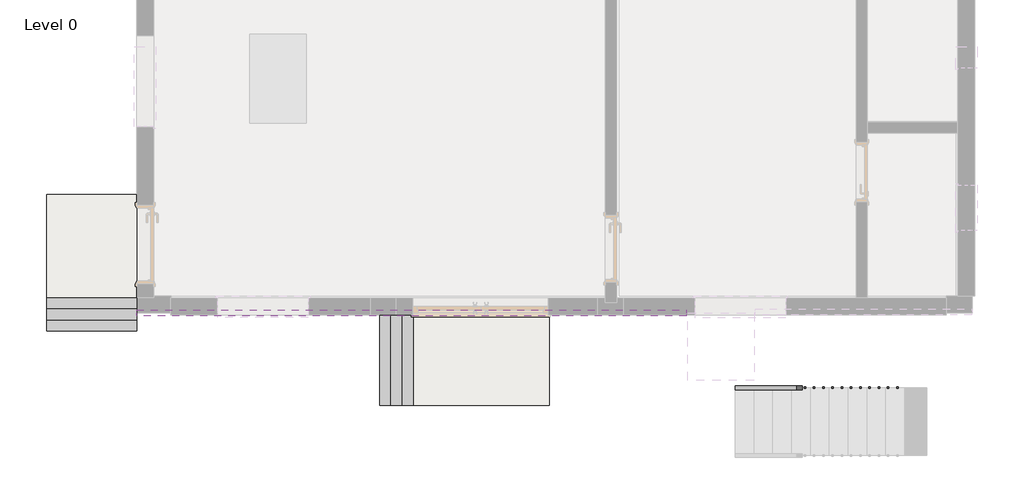
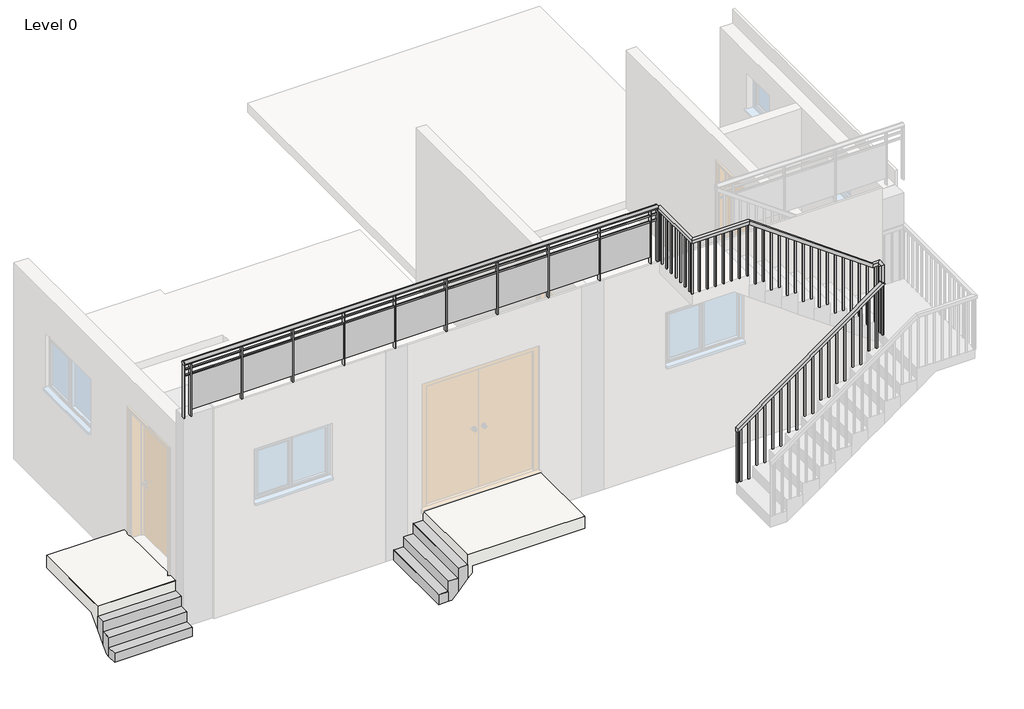
# One storey, part 2 of 3: 2 railings, 2 slabs, 2 stair flights.
"""IFC4 building model written with IfcOpenShell, lengths in millimetres."""

from ifc_helpers import new_model, si_unit, point, frame, origin, place, context, project, spatial, polyline, ellipse_curve, trimmed, outline, extrude, faceted_brep, element, save
from ifc_brep_helpers import plane_surface, extruded_surface, advanced_brep

model = new_model("IFC4")

# Units and contexts
model_context = context("Model", 3, world=origin())
ifc_project = project(units=[si_unit("LENGTHUNIT", "METRE", prefix="MILLI")], contexts=[model_context])

# Site, building, storey
site = spatial("IfcSite", under=ifc_project)
building = spatial("IfcBuilding", under=site)
storey = spatial("IfcBuildingStorey", under=building, Name="Level 0", Elevation=0.0)

# Railings
placement = place(None, origin())
element("IfcRailing", 1, ObjectType="900mm", at=placement, inside=storey, context=model_context, shape_type="SolidModel", body=[
    faceted_brep([(-2174.6019478, -2489.8095641, 610.0312421), (-2174.6019478, -2489.8095641, 548.4309995), (-2174.6019478, -2539.8095641, 548.4309995), (-2174.6019478, -2539.8095641, 610.0312421), (86.3425269, -2489.8095641, 2237.0254162), (86.3425269, -2539.8095641, 2237.0254162), (136.3425269, -2539.8095641, 2211.4055833), (136.3425269, -2489.8095641, 2211.4055833)], [[[0, 1, 2, 3]], [[4, 5, 6, 7]], [[1, 0, 4, 7]], [[2, 1, 7, 6]], [[3, 2, 6, 5]], [[0, 3, 5, 4]]]),
    faceted_brep([(86.3425269, -2513.6043721, 2237.0254162), (86.3425269, -2463.6043721, 2237.0254162), (136.3425269, -2463.6043721, 2211.4055833), (136.3425269, -2513.6043721, 2211.4055833), (86.3425269, -2513.6043721, 2509.7527012), (86.3425269, -2463.6043721, 2459.7527012), (136.3425269, -2463.6043721, 2459.7527012), (136.3425269, -2513.6043721, 2509.7527012), (86.3425269, -2438.6043721, 2509.7527012), (86.3425269, -2438.6043721, 2459.7527012), (136.3425269, -2388.6043721, 2459.7527012), (136.3425269, -2388.6043721, 2509.7527012), (11.3425269, -2438.6043721, 2509.7527012), (-4.7777331, -2438.6043721, 2459.7527012), (-4.7777331, -2388.6043721, 2459.7527012), (11.3425269, -2388.6043721, 2509.7527012), (-1920.6019478, -2438.6043721, 3900.0), (-1936.7222077, -2438.6043721, 3850.0), (-1936.7222077, -2388.6043721, 3850.0), (-1920.6019478, -2388.6043721, 3900.0), (-2838.6867445, -2438.6043721, 3900.0), (-2838.6867445, -2438.6043721, 3850.0), (-2788.6867445, -2388.6043721, 3850.0), (-2788.6867445, -2388.6043721, 3900.0), (-2838.6867445, -1501.447153, 3900.0), (-2788.6867445, -1501.447153, 3900.0), (-2788.6867445, -1501.447153, 3850.0), (-2838.6867445, -1501.447153, 3850.0)], [[[0, 1, 2, 3]], [[1, 0, 4, 5]], [[2, 1, 5, 6]], [[3, 2, 6, 7]], [[0, 3, 7, 4]], [[5, 4, 8, 9]], [[6, 5, 9, 10]], [[7, 6, 10, 11]], [[4, 7, 11, 8]], [[9, 8, 12, 13]], [[10, 9, 13, 14]], [[11, 10, 14, 15]], [[8, 11, 15, 12]], [[13, 12, 16, 17]], [[14, 13, 17, 18]], [[15, 14, 18, 19]], [[12, 15, 19, 16]], [[17, 16, 20, 21]], [[18, 17, 21, 22]], [[19, 18, 22, 23]], [[16, 19, 23, 20]], [[24, 25, 26, 27]], [[21, 20, 24, 27]], [[22, 21, 27, 26]], [[23, 22, 26, 25]], [[20, 23, 25, 24]]]),
    extrude(outline(polyline([(-2803.6867445, -1611.1043721), (-2823.6867445, -1611.1043721), (-2823.6867445, -1591.1043721), (-2803.6867445, -1591.1043721), (-2803.6867445, -1611.1043721)])), frame((0.0, 0.0, 3000.0), z_axis=(0.0, 0.0, 1.0), x_axis=(1.0, 0.0, 0.0)), (0.0, 0.0, 1.0), 850.0),
    extrude(outline(polyline([(-2803.6867445, -1736.1043721), (-2823.6867445, -1736.1043721), (-2823.6867445, -1716.1043721), (-2803.6867445, -1716.1043721), (-2803.6867445, -1736.1043721)])), frame((0.0, 0.0, 3000.0), z_axis=(0.0, 0.0, 1.0), x_axis=(1.0, 0.0, 0.0)), (0.0, 0.0, 1.0), 850.0),
    extrude(outline(polyline([(-2803.6867445, -1861.1043721), (-2823.6867445, -1861.1043721), (-2823.6867445, -1841.1043721), (-2803.6867445, -1841.1043721), (-2803.6867445, -1861.1043721)])), frame((0.0, 0.0, 3000.0), z_axis=(0.0, 0.0, 1.0), x_axis=(1.0, 0.0, 0.0)), (0.0, 0.0, 1.0), 850.0),
    extrude(outline(polyline([(-2803.6867445, -1986.1043721), (-2823.6867445, -1986.1043721), (-2823.6867445, -1966.1043721), (-2803.6867445, -1966.1043721), (-2803.6867445, -1986.1043721)])), frame((0.0, 0.0, 3000.0), z_axis=(0.0, 0.0, 1.0), x_axis=(1.0, 0.0, 0.0)), (0.0, 0.0, 1.0), 850.0),
    extrude(outline(polyline([(-2803.6867445, -2111.1043721), (-2823.6867445, -2111.1043721), (-2823.6867445, -2091.1043721), (-2803.6867445, -2091.1043721), (-2803.6867445, -2111.1043721)])), frame((0.0, 0.0, 3000.0), z_axis=(0.0, 0.0, 1.0), x_axis=(1.0, 0.0, 0.0)), (0.0, 0.0, 1.0), 850.0),
    extrude(outline(polyline([(-2803.6867445, -2236.1043721), (-2823.6867445, -2236.1043721), (-2823.6867445, -2216.1043721), (-2803.6867445, -2216.1043721), (-2803.6867445, -2236.1043721)])), frame((0.0, 0.0, 3000.0), z_axis=(0.0, 0.0, 1.0), x_axis=(1.0, 0.0, 0.0)), (0.0, 0.0, 1.0), 850.0),
    extrude(outline(polyline([(-2803.6867445, -2361.1043721), (-2823.6867445, -2361.1043721), (-2823.6867445, -2341.1043721), (-2803.6867445, -2341.1043721), (-2803.6867445, -2361.1043721)])), frame((0.0, 0.0, 3000.0), z_axis=(0.0, 0.0, 1.0), x_axis=(1.0, 0.0, 0.0)), (0.0, 0.0, 1.0), 850.0),
    extrude(outline(polyline([(-2691.1574731, -2403.6043721), (-2691.1574731, -2423.6043721), (-2711.1574731, -2423.6043721), (-2711.1574731, -2403.6043721), (-2691.1574731, -2403.6043721)])), frame((0.0, 0.0, 3000.0), z_axis=(0.0, 0.0, 1.0), x_axis=(1.0, 0.0, 0.0)), (0.0, 0.0, 1.0), 850.0),
    extrude(outline(polyline([(-2566.1574731, -2403.6043721), (-2566.1574731, -2423.6043721), (-2586.1574731, -2423.6043721), (-2586.1574731, -2403.6043721), (-2566.1574731, -2403.6043721)])), frame((0.0, 0.0, 3000.0), z_axis=(0.0, 0.0, 1.0), x_axis=(1.0, 0.0, 0.0)), (0.0, 0.0, 1.0), 850.0),
    extrude(outline(polyline([(-2441.1574731, -2403.6043721), (-2441.1574731, -2423.6043721), (-2461.1574731, -2423.6043721), (-2461.1574731, -2403.6043721), (-2441.1574731, -2403.6043721)])), frame((0.0, 0.0, 3000.0), z_axis=(0.0, 0.0, 1.0), x_axis=(1.0, 0.0, 0.0)), (0.0, 0.0, 1.0), 850.0),
    extrude(outline(polyline([(-2316.1574731, -2403.6043721), (-2316.1574731, -2423.6043721), (-2336.1574731, -2423.6043721), (-2336.1574731, -2403.6043721), (-2316.1574731, -2403.6043721)])), frame((0.0, 0.0, 3000.0), z_axis=(0.0, 0.0, 1.0), x_axis=(1.0, 0.0, 0.0)), (0.0, 0.0, 1.0), 850.0),
    extrude(outline(polyline([(-2191.1574731, -2403.6043721), (-2191.1574731, -2423.6043721), (-2211.1574731, -2423.6043721), (-2211.1574731, -2403.6043721), (-2191.1574731, -2403.6043721)])), frame((0.0, 0.0, 3000.0), z_axis=(0.0, 0.0, 1.0), x_axis=(1.0, 0.0, 0.0)), (0.0, 0.0, 1.0), 850.0),
    extrude(outline(polyline([(-2066.1574731, -2403.6043721), (-2066.1574731, -2423.6043721), (-2086.1574731, -2423.6043721), (-2086.1574731, -2403.6043721), (-2066.1574731, -2403.6043721)])), frame((0.0, 0.0, 3000.0), z_axis=(0.0, 0.0, 1.0), x_axis=(1.0, 0.0, 0.0)), (0.0, 0.0, 1.0), 850.0),
    extrude(outline(polyline([(-1941.1574731, -2403.6043721), (-1941.1574731, -2423.6043721), (-1961.1574731, -2423.6043721), (-1961.1574731, -2403.6043721), (-1941.1574731, -2403.6043721)])), frame((0.0, 0.0, 3000.0), z_axis=(0.0, 0.0, 1.0), x_axis=(1.0, 0.0, 0.0)), (0.0, 0.0, 1.0), 850.0),
    extrude(outline(polyline([(2817.2239579, -1816.1574731), (3763.2362178, -1816.1574731), (3777.6283817, -1836.1574731), (2817.2239579, -1836.1574731), (2817.2239579, -1816.1574731)])), frame((0.0, -2423.6043721, 0.0), z_axis=(0.0, 1.0, 0.0), x_axis=(0.0, 0.0, 1.0)), (0.0, 0.0, 1.0), 20.0),
    extrude(outline(polyline([(2817.2239579, -1691.1574731), (3673.2851934, -1691.1574731), (3687.6773573, -1711.1574731), (2817.2239579, -1711.1574731), (2817.2239579, -1691.1574731)])), frame((0.0, -2423.6043721, 0.0), z_axis=(0.0, 1.0, 0.0), x_axis=(0.0, 0.0, 1.0)), (0.0, 0.0, 1.0), 20.0),
    extrude(outline(polyline([(2634.4479158, -1566.1574731), (3583.3341689, -1566.1574731), (3597.7263328, -1586.1574731), (2634.4479158, -1586.1574731), (2634.4479158, -1566.1574731)])), frame((0.0, -2423.6043721, 0.0), z_axis=(0.0, 1.0, 0.0), x_axis=(0.0, 0.0, 1.0)), (0.0, 0.0, 1.0), 20.0),
    extrude(outline(polyline([(2634.4479158, -1441.1574731), (3493.3831444, -1441.1574731), (3507.7753083, -1461.1574731), (2634.4479158, -1461.1574731), (2634.4479158, -1441.1574731)])), frame((0.0, -2423.6043721, 0.0), z_axis=(0.0, 1.0, 0.0), x_axis=(0.0, 0.0, 1.0)), (0.0, 0.0, 1.0), 20.0),
    extrude(outline(polyline([(2451.6718737, -1316.1574731), (3403.43212, -1316.1574731), (3417.8242839, -1336.1574731), (2451.6718737, -1336.1574731), (2451.6718737, -1316.1574731)])), frame((0.0, -2423.6043721, 0.0), z_axis=(0.0, 1.0, 0.0), x_axis=(0.0, 0.0, 1.0)), (0.0, 0.0, 1.0), 20.0),
    extrude(outline(polyline([(2451.6718737, -1191.1574731), (3313.4810955, -1191.1574731), (3327.8732594, -1211.1574731), (2451.6718737, -1211.1574731), (2451.6718737, -1191.1574731)])), frame((0.0, -2423.6043721, 0.0), z_axis=(0.0, 1.0, 0.0), x_axis=(0.0, 0.0, 1.0)), (0.0, 0.0, 1.0), 20.0),
    extrude(outline(polyline([(2268.8958316, -1066.1574731), (3223.530071, -1066.1574731), (3237.9222349, -1086.1574731), (2268.8958316, -1086.1574731), (2268.8958316, -1066.1574731)])), frame((0.0, -2423.6043721, 0.0), z_axis=(0.0, 1.0, 0.0), x_axis=(0.0, 0.0, 1.0)), (0.0, 0.0, 1.0), 20.0),
    extrude(outline(polyline([(2268.8958316, -941.1574731), (3133.5790466, -941.1574731), (3147.9712105, -961.1574731), (2268.8958316, -961.1574731), (2268.8958316, -941.1574731)])), frame((0.0, -2423.6043721, 0.0), z_axis=(0.0, 1.0, 0.0), x_axis=(0.0, 0.0, 1.0)), (0.0, 0.0, 1.0), 20.0),
    extrude(outline(polyline([(2086.1197895, -816.1574731), (3043.6280221, -816.1574731), (3058.020186, -836.1574731), (2086.1197895, -836.1574731), (2086.1197895, -816.1574731)])), frame((0.0, -2423.6043721, 0.0), z_axis=(0.0, 1.0, 0.0), x_axis=(0.0, 0.0, 1.0)), (0.0, 0.0, 1.0), 20.0),
    extrude(outline(polyline([(2086.1197895, -691.1574731), (2953.6769976, -691.1574731), (2968.0691615, -711.1574731), (2086.1197895, -711.1574731), (2086.1197895, -691.1574731)])), frame((0.0, -2423.6043721, 0.0), z_axis=(0.0, 1.0, 0.0), x_axis=(0.0, 0.0, 1.0)), (0.0, 0.0, 1.0), 20.0),
    extrude(outline(polyline([(1903.3437474, -566.1574731), (2863.7259732, -566.1574731), (2878.1181371, -586.1574731), (1903.3437474, -586.1574731), (1903.3437474, -566.1574731)])), frame((0.0, -2423.6043721, 0.0), z_axis=(0.0, 1.0, 0.0), x_axis=(0.0, 0.0, 1.0)), (0.0, 0.0, 1.0), 20.0),
    extrude(outline(polyline([(1903.3437474, -441.1574731), (2773.7749487, -441.1574731), (2788.1671126, -461.1574731), (1903.3437474, -461.1574731), (1903.3437474, -441.1574731)])), frame((0.0, -2423.6043721, 0.0), z_axis=(0.0, 1.0, 0.0), x_axis=(0.0, 0.0, 1.0)), (0.0, 0.0, 1.0), 20.0),
    extrude(outline(polyline([(1720.5677053, -316.1574731), (2683.8239242, -316.1574731), (2698.2160881, -336.1574731), (1720.5677053, -336.1574731), (1720.5677053, -316.1574731)])), frame((0.0, -2423.6043721, 0.0), z_axis=(0.0, 1.0, 0.0), x_axis=(0.0, 0.0, 1.0)), (0.0, 0.0, 1.0), 20.0),
    extrude(outline(polyline([(1720.5677053, -191.1574731), (2593.8728998, -191.1574731), (2608.2650637, -211.1574731), (1720.5677053, -211.1574731), (1720.5677053, -191.1574731)])), frame((0.0, -2423.6043721, 0.0), z_axis=(0.0, 1.0, 0.0), x_axis=(0.0, 0.0, 1.0)), (0.0, 0.0, 1.0), 20.0),
    extrude(outline(polyline([(1537.7916632, -66.1574731), (2503.9218753, -66.1574731), (2518.3140392, -86.1574731), (1537.7916632, -86.1574731), (1537.7916632, -66.1574731)])), frame((0.0, -2423.6043721, 0.0), z_axis=(0.0, 1.0, 0.0), x_axis=(0.0, 0.0, 1.0)), (0.0, 0.0, 1.0), 20.0),
    extrude(outline(polyline([(58.8425269, -2403.6043721), (58.8425269, -2423.6043721), (38.8425269, -2423.6043721), (38.8425269, -2403.6043721), (58.8425269, -2403.6043721)])), frame((0.0, 0.0, 1537.7916632), z_axis=(0.0, 0.0, 1.0), x_axis=(1.0, 0.0, 0.0)), (0.0, 0.0, 1.0), 921.9610381),
    extrude(outline(polyline([(121.3425269, -2462.3095641), (101.3425269, -2462.3095641), (101.3425269, -2442.3095641), (121.3425269, -2442.3095641), (121.3425269, -2462.3095641)])), frame((0.0, 0.0, 1355.0156211), z_axis=(0.0, 0.0, 1.0), x_axis=(1.0, 0.0, 0.0)), (0.0, 0.0, 1.0), 1104.7370802),
    extrude(outline(polyline([(2115.3778457, 2.8980522), (1172.2395789, 2.8980522), (1172.2395789, 22.8980522), (2129.7700096, 22.8980522), (2115.3778457, 2.8980522)])), frame((0.0, -2524.8095641, 0.0), z_axis=(0.0, 1.0, 0.0), x_axis=(0.0, 0.0, 1.0)), (0.0, 0.0, 1.0), 20.0),
    extrude(outline(polyline([(2025.4268212, -122.1019478), (1172.2395789, -122.1019478), (1172.2395789, -102.1019478), (2039.8189852, -102.1019478), (2025.4268212, -122.1019478)])), frame((0.0, -2524.8095641, 0.0), z_axis=(0.0, 1.0, 0.0), x_axis=(0.0, 0.0, 1.0)), (0.0, 0.0, 1.0), 20.0),
    extrude(outline(polyline([(1935.4757968, -247.1019478), (989.4635368, -247.1019478), (989.4635368, -227.1019478), (1949.8679607, -227.1019478), (1935.4757968, -247.1019478)])), frame((0.0, -2524.8095641, 0.0), z_axis=(0.0, 1.0, 0.0), x_axis=(0.0, 0.0, 1.0)), (0.0, 0.0, 1.0), 20.0),
    extrude(outline(polyline([(1845.5247723, -372.1019478), (989.4635368, -372.1019478), (989.4635368, -352.1019478), (1859.9169362, -352.1019478), (1845.5247723, -372.1019478)])), frame((0.0, -2524.8095641, 0.0), z_axis=(0.0, 1.0, 0.0), x_axis=(0.0, 0.0, 1.0)), (0.0, 0.0, 1.0), 20.0),
    extrude(outline(polyline([(1755.5737478, -497.1019478), (806.6874947, -497.1019478), (806.6874947, -477.1019478), (1769.9659118, -477.1019478), (1755.5737478, -497.1019478)])), frame((0.0, -2524.8095641, 0.0), z_axis=(0.0, 1.0, 0.0), x_axis=(0.0, 0.0, 1.0)), (0.0, 0.0, 1.0), 20.0),
    extrude(outline(polyline([(1665.6227234, -622.1019478), (806.6874947, -622.1019478), (806.6874947, -602.1019478), (1680.0148873, -602.1019478), (1665.6227234, -622.1019478)])), frame((0.0, -2524.8095641, 0.0), z_axis=(0.0, 1.0, 0.0), x_axis=(0.0, 0.0, 1.0)), (0.0, 0.0, 1.0), 20.0),
    extrude(outline(polyline([(1575.6716989, -747.1019478), (623.9114526, -747.1019478), (623.9114526, -727.1019478), (1590.0638628, -727.1019478), (1575.6716989, -747.1019478)])), frame((0.0, -2524.8095641, 0.0), z_axis=(0.0, 1.0, 0.0), x_axis=(0.0, 0.0, 1.0)), (0.0, 0.0, 1.0), 20.0),
    extrude(outline(polyline([(1485.7206744, -872.1019478), (623.9114526, -872.1019478), (623.9114526, -852.1019478), (1500.1128384, -852.1019478), (1485.7206744, -872.1019478)])), frame((0.0, -2524.8095641, 0.0), z_axis=(0.0, 1.0, 0.0), x_axis=(0.0, 0.0, 1.0)), (0.0, 0.0, 1.0), 20.0),
    extrude(outline(polyline([(1395.76965, -997.1019478), (441.1354105, -997.1019478), (441.1354105, -977.1019478), (1410.1618139, -977.1019478), (1395.76965, -997.1019478)])), frame((0.0, -2524.8095641, 0.0), z_axis=(0.0, 1.0, 0.0), x_axis=(0.0, 0.0, 1.0)), (0.0, 0.0, 1.0), 20.0),
    extrude(outline(polyline([(1305.8186255, -1122.1019478), (441.1354105, -1122.1019478), (441.1354105, -1102.1019478), (1320.2107894, -1102.1019478), (1305.8186255, -1122.1019478)])), frame((0.0, -2524.8095641, 0.0), z_axis=(0.0, 1.0, 0.0), x_axis=(0.0, 0.0, 1.0)), (0.0, 0.0, 1.0), 20.0),
    extrude(outline(polyline([(1215.867601, -1247.1019478), (258.3593684, -1247.1019478), (258.3593684, -1227.1019478), (1230.259765, -1227.1019478), (1215.867601, -1247.1019478)])), frame((0.0, -2524.8095641, 0.0), z_axis=(0.0, 1.0, 0.0), x_axis=(0.0, 0.0, 1.0)), (0.0, 0.0, 1.0), 20.0),
    extrude(outline(polyline([(1125.9165766, -1372.1019478), (258.3593684, -1372.1019478), (258.3593684, -1352.1019478), (1140.3087405, -1352.1019478), (1125.9165766, -1372.1019478)])), frame((0.0, -2524.8095641, 0.0), z_axis=(0.0, 1.0, 0.0), x_axis=(0.0, 0.0, 1.0)), (0.0, 0.0, 1.0), 20.0),
    extrude(outline(polyline([(1035.9655521, -1497.1019478), (75.5833263, -1497.1019478), (75.5833263, -1477.1019478), (1050.357716, -1477.1019478), (1035.9655521, -1497.1019478)])), frame((0.0, -2524.8095641, 0.0), z_axis=(0.0, 1.0, 0.0), x_axis=(0.0, 0.0, 1.0)), (0.0, 0.0, 1.0), 20.0),
    extrude(outline(polyline([(946.0145276, -1622.1019478), (75.5833263, -1622.1019478), (75.5833263, -1602.1019478), (960.4066916, -1602.1019478), (946.0145276, -1622.1019478)])), frame((0.0, -2524.8095641, 0.0), z_axis=(0.0, 1.0, 0.0), x_axis=(0.0, 0.0, 1.0)), (0.0, 0.0, 1.0), 20.0),
    extrude(outline(polyline([(856.0635032, -1747.1019478), (-107.1927158, -1747.1019478), (-107.1927158, -1727.1019478), (870.4556671, -1727.1019478), (856.0635032, -1747.1019478)])), frame((0.0, -2524.8095641, 0.0), z_axis=(0.0, 1.0, 0.0), x_axis=(0.0, 0.0, 1.0)), (0.0, 0.0, 1.0), 20.0),
    extrude(outline(polyline([(766.1124787, -1872.1019478), (-107.1927158, -1872.1019478), (-107.1927158, -1852.1019478), (780.5046426, -1852.1019478), (766.1124787, -1872.1019478)])), frame((0.0, -2524.8095641, 0.0), z_axis=(0.0, 1.0, 0.0), x_axis=(0.0, 0.0, 1.0)), (0.0, 0.0, 1.0), 20.0),
    extrude(outline(polyline([(676.1614542, -1997.1019478), (-289.9687579, -1997.1019478), (-289.9687579, -1977.1019478), (690.5536182, -1977.1019478), (676.1614542, -1997.1019478)])), frame((0.0, -2524.8095641, 0.0), z_axis=(0.0, 1.0, 0.0), x_axis=(0.0, 0.0, 1.0)), (0.0, 0.0, 1.0), 20.0),
    extrude(outline(polyline([(586.2104298, -2122.1019478), (-289.9687579, -2122.1019478), (-289.9687579, -2102.1019478), (600.6025937, -2102.1019478), (586.2104298, -2122.1019478)])), frame((0.0, -2524.8095641, 0.0), z_axis=(0.0, 1.0, 0.0), x_axis=(0.0, 0.0, 1.0)), (0.0, 0.0, 1.0), 20.0),
    extrude(outline(polyline([(-2803.6867445, -2403.6043721), (-2803.6867445, -2423.6043721), (-2823.6867445, -2423.6043721), (-2823.6867445, -2403.6043721), (-2803.6867445, -2403.6043721)])), frame((0.0, 0.0, 3000.0), z_axis=(0.0, 0.0, 1.0), x_axis=(1.0, 0.0, 0.0)), (0.0, 0.0, 1.0), 850.0),
    extrude(outline(polyline([(121.3425269, -2423.6043721), (101.3425269, -2423.6043721), (101.3425269, -2403.6043721), (121.3425269, -2403.6043721), (121.3425269, -2423.6043721)])), frame((0.0, 0.0, 1355.0156211), z_axis=(0.0, 0.0, 1.0), x_axis=(1.0, 0.0, 0.0)), (0.0, 0.0, 1.0), 1104.7370802),
    extrude(outline(polyline([(2186.2192965, 101.3425269), (1355.0156211, 101.3425269), (1355.0156211, 121.3425269), (2200.6114604, 121.3425269), (2186.2192965, 101.3425269)])), frame((0.0, -2524.8095641, 0.0), z_axis=(0.0, 1.0, 0.0), x_axis=(0.0, 0.0, 1.0)), (0.0, 0.0, 1.0), 20.0),
    extrude(outline(polyline([(-2803.6867445, -1521.447153), (-2823.6867445, -1521.447153), (-2823.6867445, -1501.447153), (-2803.6867445, -1501.447153), (-2803.6867445, -1521.447153)])), frame((0.0, 0.0, 3000.0), z_axis=(0.0, 0.0, 1.0), x_axis=(1.0, 0.0, 0.0)), (0.0, 0.0, 1.0), 850.0),
    extrude(outline(polyline([(548.4309995, -2174.6019478), (-289.9687579, -2174.6019478), (-289.9687579, -2154.6019478), (562.8231634, -2154.6019478), (548.4309995, -2174.6019478)])), frame((0.0, -2524.8095641, 0.0), z_axis=(0.0, 1.0, 0.0), x_axis=(0.0, 0.0, 1.0)), (0.0, 0.0, 1.0), 20.0),
])
element("IfcRailing", 2, ObjectType="Glass_Panel-Bottom_Fill", at=placement, inside=storey, context=model_context, shape_type="SolidModel", body=[
    advanced_brep(
    [(-10252.3493191, -1462.0563878, 3900.0), (-10252.3493191, -1502.0563878, 3870.0), (-10252.3493191, -1542.0563878, 3900.0), (-10252.3493191, -1502.0563878, 3930.0), (-2838.6867445, -1462.0563878, 3900.0), (-2838.6867445, -1502.0563878, 3930.0), (-2838.6867445, -1542.0563878, 3900.0), (-2838.6867445, -1502.0563878, 3870.0)],
    [
        (0, 1, ellipse_curve(frame((-10252.3493191, -1502.0563878, 3900.0), z_axis=(-1.0, 0.0, 0.0), x_axis=(0.0, -1.0, 0.0)), 40.0, 30.0)),
        (1, 2, ellipse_curve(frame((-10252.3493191, -1502.0563878, 3900.0), z_axis=(-1.0, 0.0, 0.0), x_axis=(0.0, -1.0, 0.0)), 40.0, 30.0)),
        (2, 3, ellipse_curve(frame((-10252.3493191, -1502.0563878, 3900.0), z_axis=(-1.0, 0.0, 0.0), x_axis=(0.0, -1.0, 0.0)), 40.0, 30.0)),
        (3, 0, ellipse_curve(frame((-10252.3493191, -1502.0563878, 3900.0), z_axis=(-1.0, 0.0, 0.0), x_axis=(0.0, -1.0, 0.0)), 40.0, 30.0)),
        (4, 5, ellipse_curve(frame((-2838.6867445, -1502.0563878, 3900.0), z_axis=(1.0, 0.0, 0.0), x_axis=(0.0, -1.0, 0.0)), 40.0, 30.0)),
        (5, 6, ellipse_curve(frame((-2838.6867445, -1502.0563878, 3900.0), z_axis=(1.0, 0.0, 0.0), x_axis=(0.0, -1.0, 0.0)), 40.0, 30.0)),
        (6, 7, ellipse_curve(frame((-2838.6867445, -1502.0563878, 3900.0), z_axis=(1.0, 0.0, 0.0), x_axis=(0.0, -1.0, 0.0)), 40.0, 30.0)),
        (7, 4, ellipse_curve(frame((-2838.6867445, -1502.0563878, 3900.0), z_axis=(1.0, 0.0, 0.0), x_axis=(0.0, -1.0, 0.0)), 40.0, 30.0)),
        (0, 4),
        (7, 1),
        (6, 2),
        (5, 3),
    ],
    [
        plane_surface(frame((-10252.3493191, -1502.0563878, 3900.0), z_axis=(-1.0, 0.0, 0.0), x_axis=(0.0, 1.0, 0.0))),
        plane_surface(frame((-2838.6867445, -1502.0563878, 3900.0), z_axis=(1.0, 0.0, 0.0), x_axis=(0.0, 1.0, 0.0))),
        extruded_surface(trimmed(ellipse_curve(frame((-2838.6867445, -1502.0563878, 3900.0), z_axis=(-1.0, 0.0, 0.0), x_axis=(0.0, -1.0, 0.0)), 40.0, 30.0), [point((-2838.6867445, -1462.0563878, 3900.0))], [point((-2838.6867445, -1502.0563878, 3870.0))], True, "CARTESIAN"), (-7413.6625746, 0.0, 0.0), 7413.6625746),
        extruded_surface(trimmed(ellipse_curve(frame((-2838.6867445, -1502.0563878, 3900.0), z_axis=(-1.0, 0.0, 0.0), x_axis=(0.0, -1.0, 0.0)), 40.0, 30.0), [point((-2838.6867445, -1502.0563878, 3870.0))], [point((-2838.6867445, -1542.0563878, 3900.0))], True, "CARTESIAN"), (-7413.6625746, 0.0, 0.0), 7413.6625746),
        extruded_surface(trimmed(ellipse_curve(frame((-2838.6867445, -1502.0563878, 3900.0), z_axis=(-1.0, 0.0, 0.0), x_axis=(0.0, -1.0, 0.0)), 40.0, 30.0), [point((-2838.6867445, -1542.0563878, 3900.0))], [point((-2838.6867445, -1502.0563878, 3930.0))], True, "CARTESIAN"), (-7413.6625746, 0.0, 0.0), 7413.6625746),
        extruded_surface(trimmed(ellipse_curve(frame((-2838.6867445, -1502.0563878, 3900.0), z_axis=(-1.0, 0.0, 0.0), x_axis=(0.0, -1.0, 0.0)), 40.0, 30.0), [point((-2838.6867445, -1502.0563878, 3930.0))], [point((-2838.6867445, -1462.0563878, 3900.0))], True, "CARTESIAN"), (-7413.6625746, 0.0, 0.0), 7413.6625746),
    ],
    [
        (0, [[1, 2, 3, 4]]),
        (1, [[5, 6, 7, 8]]),
        (2, [[-1, 9, -8, 10]]),
        (3, [[-2, -10, -7, 11]]),
        (4, [[-3, -11, -6, 12]]),
        (5, [[-4, -12, -5, -9]]),
    ],
),
    extrude(outline(polyline([(-10252.3493191, -1511.447153), (-10252.3493191, -1491.447153), (-2838.6867445, -1491.447153), (-2838.6867445, -1511.447153), (-10252.3493191, -1511.447153)])), frame((0.0, 0.0, 3780.0), z_axis=(0.0, 0.0, 1.0), x_axis=(1.0, 0.0, 0.0)), (0.0, 0.0, 1.0), 20.0),
    extrude(outline(polyline([(-10252.3493191, -1511.447153), (-10252.3493191, -1491.447153), (-2838.6867445, -1491.447153), (-2838.6867445, -1511.447153), (-10252.3493191, -1511.447153)])), frame((0.0, 0.0, 3680.0), z_axis=(0.0, 0.0, 1.0), x_axis=(1.0, 0.0, 0.0)), (0.0, 0.0, 1.0), 20.0),
    extrude(outline(polyline([(-2951.5180318, -1476.447153), (-2939.5180318, -1476.447153), (-2939.5180318, -1526.447153), (-2951.5180318, -1526.447153), (-2951.5180318, -1476.447153)])), frame((0.0, 0.0, 3000.0), z_axis=(0.0, 0.0, 1.0), x_axis=(1.0, 0.0, 0.0)), (0.0, 0.0, 1.0), 870.0),
    extrude(outline(polyline([(-3745.5180318, -1503.171963), (-2945.5180318, -1503.171963), (-2945.5180318, -1508.171963), (-3745.5180318, -1508.171963), (-3745.5180318, -1503.171963)])), frame((0.0, 0.0, 3100.0), z_axis=(0.0, 0.0, 1.0), x_axis=(1.0, 0.0, 0.0)), (0.0, 0.0, 1.0), 600.0),
    extrude(outline(polyline([(-3751.5180318, -1476.447153), (-3739.5180318, -1476.447153), (-3739.5180318, -1526.447153), (-3751.5180318, -1526.447153), (-3751.5180318, -1476.447153)])), frame((0.0, 0.0, 3000.0), z_axis=(0.0, 0.0, 1.0), x_axis=(1.0, 0.0, 0.0)), (0.0, 0.0, 1.0), 870.0),
    extrude(outline(polyline([(-4545.5180318, -1503.171963), (-3745.5180318, -1503.171963), (-3745.5180318, -1508.171963), (-4545.5180318, -1508.171963), (-4545.5180318, -1503.171963)])), frame((0.0, 0.0, 3100.0), z_axis=(0.0, 0.0, 1.0), x_axis=(1.0, 0.0, 0.0)), (0.0, 0.0, 1.0), 600.0),
    extrude(outline(polyline([(-4551.5180318, -1476.447153), (-4539.5180318, -1476.447153), (-4539.5180318, -1526.447153), (-4551.5180318, -1526.447153), (-4551.5180318, -1476.447153)])), frame((0.0, 0.0, 3000.0), z_axis=(0.0, 0.0, 1.0), x_axis=(1.0, 0.0, 0.0)), (0.0, 0.0, 1.0), 870.0),
    extrude(outline(polyline([(-5345.5180318, -1503.171963), (-4545.5180318, -1503.171963), (-4545.5180318, -1508.171963), (-5345.5180318, -1508.171963), (-5345.5180318, -1503.171963)])), frame((0.0, 0.0, 3100.0), z_axis=(0.0, 0.0, 1.0), x_axis=(1.0, 0.0, 0.0)), (0.0, 0.0, 1.0), 600.0),
    extrude(outline(polyline([(-5351.5180318, -1476.447153), (-5339.5180318, -1476.447153), (-5339.5180318, -1526.447153), (-5351.5180318, -1526.447153), (-5351.5180318, -1476.447153)])), frame((0.0, 0.0, 3000.0), z_axis=(0.0, 0.0, 1.0), x_axis=(1.0, 0.0, 0.0)), (0.0, 0.0, 1.0), 870.0),
    extrude(outline(polyline([(-6145.5180318, -1503.171963), (-5345.5180318, -1503.171963), (-5345.5180318, -1508.171963), (-6145.5180318, -1508.171963), (-6145.5180318, -1503.171963)])), frame((0.0, 0.0, 3100.0), z_axis=(0.0, 0.0, 1.0), x_axis=(1.0, 0.0, 0.0)), (0.0, 0.0, 1.0), 600.0),
    extrude(outline(polyline([(-6151.5180318, -1476.447153), (-6139.5180318, -1476.447153), (-6139.5180318, -1526.447153), (-6151.5180318, -1526.447153), (-6151.5180318, -1476.447153)])), frame((0.0, 0.0, 3000.0), z_axis=(0.0, 0.0, 1.0), x_axis=(1.0, 0.0, 0.0)), (0.0, 0.0, 1.0), 870.0),
    extrude(outline(polyline([(-6945.5180318, -1503.171963), (-6145.5180318, -1503.171963), (-6145.5180318, -1508.171963), (-6945.5180318, -1508.171963), (-6945.5180318, -1503.171963)])), frame((0.0, 0.0, 3100.0), z_axis=(0.0, 0.0, 1.0), x_axis=(1.0, 0.0, 0.0)), (0.0, 0.0, 1.0), 600.0),
    extrude(outline(polyline([(-6951.5180318, -1476.447153), (-6939.5180318, -1476.447153), (-6939.5180318, -1526.447153), (-6951.5180318, -1526.447153), (-6951.5180318, -1476.447153)])), frame((0.0, 0.0, 3000.0), z_axis=(0.0, 0.0, 1.0), x_axis=(1.0, 0.0, 0.0)), (0.0, 0.0, 1.0), 870.0),
    extrude(outline(polyline([(-7745.5180318, -1503.171963), (-6945.5180318, -1503.171963), (-6945.5180318, -1508.171963), (-7745.5180318, -1508.171963), (-7745.5180318, -1503.171963)])), frame((0.0, 0.0, 3100.0), z_axis=(0.0, 0.0, 1.0), x_axis=(1.0, 0.0, 0.0)), (0.0, 0.0, 1.0), 600.0),
    extrude(outline(polyline([(-7751.5180318, -1476.447153), (-7739.5180318, -1476.447153), (-7739.5180318, -1526.447153), (-7751.5180318, -1526.447153), (-7751.5180318, -1476.447153)])), frame((0.0, 0.0, 3000.0), z_axis=(0.0, 0.0, 1.0), x_axis=(1.0, 0.0, 0.0)), (0.0, 0.0, 1.0), 870.0),
    extrude(outline(polyline([(-8545.5180318, -1503.171963), (-7745.5180318, -1503.171963), (-7745.5180318, -1508.171963), (-8545.5180318, -1508.171963), (-8545.5180318, -1503.171963)])), frame((0.0, 0.0, 3100.0), z_axis=(0.0, 0.0, 1.0), x_axis=(1.0, 0.0, 0.0)), (0.0, 0.0, 1.0), 600.0),
    extrude(outline(polyline([(-8551.5180318, -1476.447153), (-8539.5180318, -1476.447153), (-8539.5180318, -1526.447153), (-8551.5180318, -1526.447153), (-8551.5180318, -1476.447153)])), frame((0.0, 0.0, 3000.0), z_axis=(0.0, 0.0, 1.0), x_axis=(1.0, 0.0, 0.0)), (0.0, 0.0, 1.0), 870.0),
    extrude(outline(polyline([(-9345.5180318, -1503.171963), (-8545.5180318, -1503.171963), (-8545.5180318, -1508.171963), (-9345.5180318, -1508.171963), (-9345.5180318, -1503.171963)])), frame((0.0, 0.0, 3100.0), z_axis=(0.0, 0.0, 1.0), x_axis=(1.0, 0.0, 0.0)), (0.0, 0.0, 1.0), 600.0),
    extrude(outline(polyline([(-9351.5180318, -1476.447153), (-9339.5180318, -1476.447153), (-9339.5180318, -1526.447153), (-9351.5180318, -1526.447153), (-9351.5180318, -1476.447153)])), frame((0.0, 0.0, 3000.0), z_axis=(0.0, 0.0, 1.0), x_axis=(1.0, 0.0, 0.0)), (0.0, 0.0, 1.0), 870.0),
    extrude(outline(polyline([(-10145.5180318, -1503.171963), (-9345.5180318, -1503.171963), (-9345.5180318, -1508.171963), (-10145.5180318, -1508.171963), (-10145.5180318, -1503.171963)])), frame((0.0, 0.0, 3100.0), z_axis=(0.0, 0.0, 1.0), x_axis=(1.0, 0.0, 0.0)), (0.0, 0.0, 1.0), 600.0),
    extrude(outline(polyline([(-10151.5180318, -1476.447153), (-10139.5180318, -1476.447153), (-10139.5180318, -1526.447153), (-10151.5180318, -1526.447153), (-10151.5180318, -1476.447153)])), frame((0.0, 0.0, 3000.0), z_axis=(0.0, 0.0, 1.0), x_axis=(1.0, 0.0, 0.0)), (0.0, 0.0, 1.0), 870.0),
    extrude(outline(polyline([(-2846.6867445, -1476.447153), (-2834.6867445, -1476.447153), (-2834.6867445, -1526.447153), (-2846.6867445, -1526.447153), (-2846.6867445, -1476.447153)])), frame((0.0, 0.0, 3000.0), z_axis=(0.0, 0.0, 1.0), x_axis=(1.0, 0.0, 0.0)), (0.0, 0.0, 1.0), 870.0),
    extrude(outline(polyline([(-10256.3493191, -1476.447153), (-10244.3493191, -1476.447153), (-10244.3493191, -1526.447153), (-10256.3493191, -1526.447153), (-10256.3493191, -1476.447153)])), frame((0.0, 0.0, 3000.0), z_axis=(0.0, 0.0, 1.0), x_axis=(1.0, 0.0, 0.0)), (0.0, 0.0, 1.0), 870.0),
])

# Slabs
element("IfcSlab", 3, ObjectType="200mm_Thickness", at=placement, inside=storey, context=model_context, shape_type="SolidModel", body=[
    faceted_brep([(-6517.9703754, -1528.9995449, 175.64), (-6517.9703754, -2748.1843061, 175.64), (-4689.2045313, -2748.1843061, 175.64), (-4689.2045313, -1528.9995449, 175.64), (-4689.2045313, -2748.1843061, -24.36), (-4689.2045313, -1528.9995449, -24.36), (-6452.7425878, -1528.9995449, -24.36), (-6452.7425878, -1528.9995449, -140.44), (-6517.9703754, -1528.9995449, -211.6147869), (-6517.9703754, -1528.9995449, -24.36), (-6517.9703754, -1528.9995449, 9.56), (-6517.9703754, -2748.1843061, 9.56), (-6517.9703754, -2748.1843061, -24.36), (-6517.9703754, -2748.1843061, -211.6147869), (-6452.7425878, -2748.1843061, -140.44), (-6452.7425878, -2748.1843061, -24.36)], [[[0, 1, 2, 3]], [[3, 2, 4, 5]], [[0, 3, 5, 6, 7, 8, 9, 10]], [[2, 1, 11, 12, 13, 14, 15, 4]], [[1, 0, 10, 9, 8, 13, 12, 11]], [[15, 6, 5, 4]], [[7, 14, 13, 8]], [[14, 7, 6, 15]]]),
    extrude(outline(polyline([(-6517.9703754, -1528.9995449), (-4689.2045313, -1528.9995449), (-4689.2045313, -2748.1843061), (-6517.9703754, -2748.1843061), (-6517.9703754, -1528.9995449)])), frame((0.0, 0.0, 175.64), z_axis=(0.0, 0.0, 1.0), x_axis=(1.0, 0.0, 0.0)), (0.0, 0.0, 1.0), 1.0),
])
element("IfcSlab", 4, ObjectType="200mm_Thickness", at=placement, inside=storey, context=model_context, shape_type="SolidModel", body=[
    faceted_brep([(-11471.5114848, -1290.9249414, 175.64), (-10252.3493191, -1290.9249414, 175.64), (-10252.3493191, -1118.5479552, 175.64), (-10252.3493191, 96.9125444, 175.64), (-11471.5114848, 96.9125444, 175.64), (-11471.5114848, -1118.5479552, 175.64), (-11471.5114848, -1290.9249414, -212.4530767), (-11471.5114848, -1290.9249414, 9.56), (-11471.5114848, 96.9125444, -24.36), (-11471.5114848, -1118.5479552, -24.36), (-10252.3493191, -1290.9249414, 9.56), (-10252.3493191, -1290.9249414, -212.4530767), (-10252.3493191, -1118.5479552, -24.36), (-10252.3493191, 96.9125444, -24.36)], [[[0, 1, 2, 3, 4, 5]], [[6, 7, 0, 5, 4, 8, 9]], [[1, 10, 11, 12, 13, 3, 2]], [[4, 3, 13, 8]], [[1, 0, 7, 6, 11, 10]], [[12, 9, 8, 13]], [[9, 12, 11, 6]]]),
    extrude(outline(polyline([(-11471.5114848, -1290.9249414), (-11471.5114848, 96.9125444), (-10252.3493191, 96.9125444), (-10252.3493191, -1290.9249414), (-11471.5114848, -1290.9249414)])), frame((0.0, 0.0, 175.64), z_axis=(0.0, 0.0, 1.0), x_axis=(1.0, 0.0, 0.0)), (0.0, 0.0, 1.0), 1.0),
])

# Stair flights
element("IfcStairFlight", 5, ObjectType="1mm_Tread-150mm_Depth", at=placement, inside=storey, context=model_context, shape_type="SolidModel", body=[
    faceted_brep([(-6823.1450401, -1528.9995449, -322.6), (-6975.3482492, -1528.9995449, -322.6), (-6975.3482492, -2748.1843061, -322.6), (-6823.1450401, -2748.1843061, -322.6), (-6823.1450401, -1528.9995449, -487.68), (-6975.3482492, -1528.9995449, -487.68), (-6975.3482492, -2748.1843061, -487.68), (-6823.1450401, -2748.1843061, -487.68), (-6670.941831, -1528.9995449, -156.52), (-6823.1450401, -1528.9995449, -156.52), (-6823.1450401, -2748.1843061, -156.52), (-6670.941831, -2748.1843061, -156.52), (-6670.941831, -1528.9995449, -378.5330767), (-6770.9689986, -1528.9995449, -487.68), (-6770.9689986, -2748.1843061, -487.68), (-6670.941831, -2748.1843061, -378.5330767), (-6517.9703754, -1528.9995449, 9.56), (-6670.941831, -1528.9995449, 9.56), (-6670.941831, -2748.1843061, 9.56), (-6517.9703754, -2748.1843061, 9.56), (-6517.9703754, -1528.9995449, -211.6147869), (-6517.9703754, -2748.1843061, -211.6147869)], [[[0, 1, 2, 3]], [[1, 0, 4, 5]], [[2, 1, 5, 6]], [[3, 2, 6, 7]], [[8, 9, 10, 11]], [[4, 0, 9, 8, 12, 13]], [[0, 3, 10, 9]], [[3, 7, 14, 15, 11, 10]], [[16, 17, 18, 19]], [[17, 16, 20, 12, 8]], [[8, 11, 18, 17]], [[19, 18, 11, 15, 21]], [[16, 19, 21, 20]], [[5, 4, 13, 14, 7, 6]], [[14, 13, 12, 20, 21, 15]]]),
    extrude(outline(polyline([(-6823.1450401, -1528.9995449), (-6823.1450401, -2748.1843061), (-6975.3482492, -2748.1843061), (-6975.3482492, -1528.9995449), (-6823.1450401, -1528.9995449)])), frame((0.0, 0.0, -322.6), z_axis=(0.0, 0.0, 1.0), x_axis=(1.0, 0.0, 0.0)), (0.0, 0.0, 1.0), 1.0),
    extrude(outline(polyline([(-6670.941831, -1528.9995449), (-6670.941831, -2748.1843061), (-6823.1450401, -2748.1843061), (-6823.1450401, -1528.9995449), (-6670.941831, -1528.9995449)])), frame((0.0, 0.0, -156.52), z_axis=(0.0, 0.0, 1.0), x_axis=(1.0, 0.0, 0.0)), (0.0, 0.0, 1.0), 1.0),
    extrude(outline(polyline([(-6517.9703754, -1528.9995449), (-6517.9703754, -2748.1843061), (-6670.941831, -2748.1843061), (-6670.941831, -1528.9995449), (-6517.9703754, -1528.9995449)])), frame((0.0, 0.0, 9.56), z_axis=(0.0, 0.0, 1.0), x_axis=(1.0, 0.0, 0.0)), (0.0, 0.0, 1.0), 1.0),
])
element("IfcStairFlight", 6, ObjectType="1mm_Tread-150mm_Depth", at=placement, inside=storey, context=model_context, shape_type="SolidModel", body=[
    faceted_brep([(-11471.5114848, -1595.3313595, -322.6), (-11471.5114848, -1748.3254106, -322.6), (-10252.3493191, -1748.3254106, -322.6), (-10252.3493191, -1595.3313595, -322.6), (-11471.5114848, -1595.3313595, -472.6), (-11471.5114848, -1748.3254106, -472.6), (-10252.3493191, -1748.3254106, -472.6), (-10252.3493191, -1595.3313595, -472.6), (-11471.5114848, -1595.3313595, -156.52), (-10252.3493191, -1595.3313595, -156.52), (-10252.3493191, -1529.3353253, -156.52), (-10252.3493191, -1443.1281504, -156.52), (-11471.5114848, -1443.1281504, -156.52), (-11471.5114848, -1529.3353253, -156.52), (-11471.5114848, -1443.1281504, -378.5330767), (-11471.5114848, -1529.3353253, -472.6), (-10252.3493191, -1529.3353253, -472.6), (-10252.3493191, -1443.1281504, -378.5330767), (-11471.5114848, -1290.9249414, 9.56), (-11471.5114848, -1443.1281504, 9.56), (-10252.3493191, -1443.1281504, 9.56), (-10252.3493191, -1290.9249414, 9.56), (-11471.5114848, -1290.9249414, -212.4530767), (-10252.3493191, -1290.9249414, -212.4530767)], [[[0, 1, 2, 3]], [[1, 0, 4, 5]], [[2, 1, 5, 6]], [[3, 2, 6, 7]], [[8, 9, 10, 11, 12, 13]], [[0, 8, 13, 12, 14, 15, 4]], [[0, 3, 9, 8]], [[9, 3, 7, 16, 17, 11, 10]], [[18, 19, 20, 21]], [[19, 18, 22, 14, 12]], [[12, 11, 20, 19]], [[21, 20, 11, 17, 23]], [[18, 21, 23, 22]], [[15, 16, 7, 6, 5, 4]], [[16, 15, 14, 22, 23, 17]]]),
    extrude(outline(polyline([(-11471.5114848, -1595.3313595), (-10252.3493191, -1595.3313595), (-10252.3493191, -1748.3254106), (-11471.5114848, -1748.3254106), (-11471.5114848, -1595.3313595)])), frame((0.0, 0.0, -322.6), z_axis=(0.0, 0.0, 1.0), x_axis=(1.0, 0.0, 0.0)), (0.0, 0.0, 1.0), 1.0),
    extrude(outline(polyline([(-11471.5114848, -1443.1281504), (-10252.3493191, -1443.1281504), (-10252.3493191, -1595.3313595), (-11471.5114848, -1595.3313595), (-11471.5114848, -1443.1281504)])), frame((0.0, 0.0, -156.52), z_axis=(0.0, 0.0, 1.0), x_axis=(1.0, 0.0, 0.0)), (0.0, 0.0, 1.0), 1.0),
    extrude(outline(polyline([(-11471.5114848, -1290.9249414), (-10252.3493191, -1290.9249414), (-10252.3493191, -1443.1281504), (-11471.5114848, -1443.1281504), (-11471.5114848, -1290.9249414)])), frame((0.0, 0.0, 9.56), z_axis=(0.0, 0.0, 1.0), x_axis=(1.0, 0.0, 0.0)), (0.0, 0.0, 1.0), 1.0),
])

save(model, "model.ifc")

# Revit data of these elements
# Type "900mm"
#   built-in parameter 1008612 = 0.019685 (stored number, unit not read)
#   built-in parameter 1008611 = 0.019685 (stored number, unit not read)
#   built-in parameter 1008609 = 0.902231 (stored number, unit not read)
#   built-in parameter 1008604 = 0.19685 (stored number, unit not read)
#   built-in parameter 1008603 = 0.164042 (stored number, unit not read)
#   Railing Height = 2.952756 ft
#   built-in parameter 1008630 = 2
#   built-in parameter 1008610 = 2
#   built-in parameter 1008608 = 1
#   built-in parameter 1008618 = Baluster_Square : 20mm
# Type "Glass_Panel-Bottom_Fill"
#   built-in parameter 1008612 = 0.019685 (stored number, unit not read)
#   built-in parameter 1008611 = 0.019685 (stored number, unit not read)
#   built-in parameter 1008609 = 0.902231 (stored number, unit not read)
#   built-in parameter 1008604 = 0.19685 (stored number, unit not read)
#   built-in parameter 1008603 = 0.164042 (stored number, unit not read)
#   Railing Height = 2.952756 ft
#   built-in parameter 1008630 = 2
#   built-in parameter 1008610 = 2
# Element 1 (IfcRailing, "900mm")
#   Phase Created = New Construction
# Element 2 (IfcRailing, "Glass_Panel-Bottom_Fill")
#   Phase Created = New Construction
#   Materials on its faces: "Metal - Stainless Steel,Polished", "Glass"
# Elements 3, 4 (IfcSlab, "200mm_Thickness")
#   Phase Created = New Construction
#   Materials on its faces: "Concrete, Cast-in-Place gray"
# Elements 5, 6 (IfcStairFlight, "1mm_Tread-150mm_Depth")
#   Phase Created = New Construction
#   Materials on its faces: "Concrete, Cast-in-Place gray"
# Materials
#   "Metal - Stainless Steel,Polished": class "Metal", colour RGB 236 239 239, transparency 0, Cost = 0
#   "Glass": class "Glass", colour RGB 0 128 192, transparency 0.9, Description = "Soda Lime Glass", Cost = 0
#   "Concrete, Cast-in-Place gray": class "Concrete", colour RGB 192 192 192, transparency 0, Description = "Cast-in-place concrete", Cost = 0
